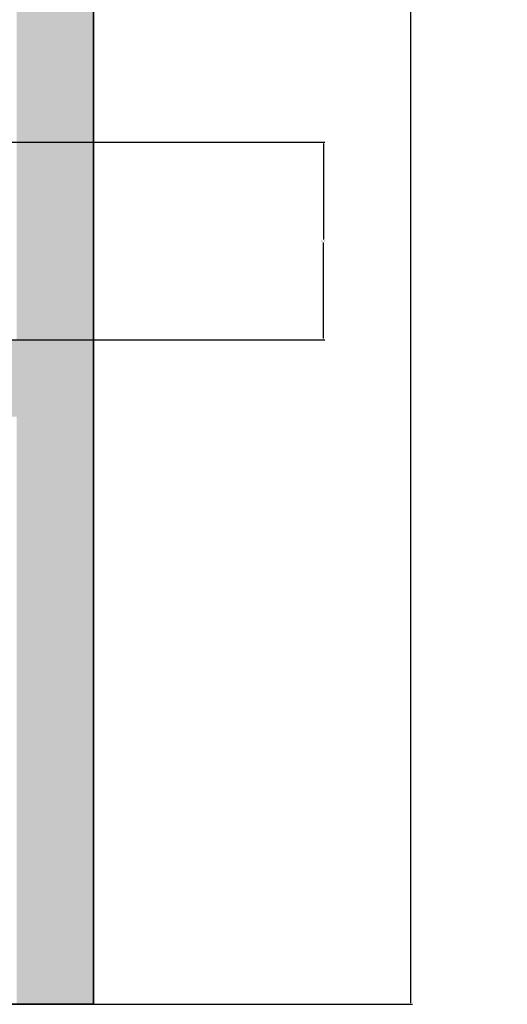
# Model space of a CAD drawing. Units: inches. Extents: x -5 to 330, y -522 to 40.
# Tile 18 of 23: x 272 to 330, y -495 to -380. Entities that reach past the tile are written whole.
import ezdxf

# ---------------------------------------------------------------- set-up
doc = ezdxf.new("R2010")
doc.units = ezdxf.units.IN
doc.header["$MEASUREMENT"] = 0
for name, color, linetype, lineweight in [('A-ANNO-DIMS', 2, 'Continuous', 18), ('A-SITE-WALL', 7, 'Continuous', 35), ('A-WALL', 7, 'Continuous', 35)]:
    doc.layers.add(name, color=color, linetype=linetype, lineweight=lineweight)
doc.layers.add('A-WALL-PATT', color=18, linetype='Continuous', lineweight=13, true_color=0x000000)
doc.styles.get("Standard").update_dxf_attribs({"font": 'arial.ttf'})
doc.dimstyles.get("Standard").update_dxf_attribs({"dimtxt": 0.18, "dimasz": 0.18, "dimexe": 0.18, "dimexo": 0.0625, "dimgap": 0.09, "dimtad": 0, "dimtih": 1, "dimtoh": 1, "dimdec": 0, "dimzin": 0, "dimdsep": 46, "dimlunit": 3, "dimtxsty": 'Standard', "dimcen": 0.09, "dimadec": 0, "dimazin": 0, "dimtfac": 1, "dimtdec": 0, "dimtofl": 0, "dimtmove": 0, "dimatfit": 3, "dimfxl": 1, "dimtolj": 1, "dimtzin": 0, "dimarcsym": 0})

# ---------------------------------------------------------------- blocks, each defined once
blk = doc.blocks.new('*D6')
at = {"layer": 'A-ANNO-DIMS', "color": 0, "lineweight": -2, "transparency": 16777216}
for p, q in [((281.07, 12.36), (318.43, 12.36)), ((318.25, 12.18), (318.25, -238.29)), ((318.25, -494.96), (318.25, -244.5)), ((281.07, -495.14), (318.43, -495.14))]:
    blk.add_line(p, q, dxfattribs=at)
at = {"layer": 'A-ANNO-DIMS', "color": 0, "transparency": 16777216}
for points in [[(318.22, 12.18), (318.28, 12.18), (318.25, 12.36)], [(318.22, -494.96), (318.28, -494.96), (318.25, -495.14)]]:
    blk.add_solid(points, dxfattribs=at)
at = {"layer": 'Defpoints', "color": 0, "transparency": 16777216}
for p in [(281.01, 12.36), (281.01, -495.14), (318.25, -495.14)]:
    blk.add_point(p, dxfattribs=at)
at = {"layer": 'A-ANNO-DIMS', "color": 0, "transparency": 16777216, "insert": (318.25, -241.39), "char_height": 6, "attachment_point": 5}
blk.add_mtext('\\A1;42\'-4"', dxfattribs=at)
blk = doc.blocks.new('*D44')
at = {"layer": 'A-ANNO-DIMS', "color": 0, "lineweight": -2, "transparency": 16777216}
for p, q in [((128.57, -393.93), (308.17, -393.93)), ((307.99, -394.11), (307.99, -405.36)), ((307.99, -416.96), (307.99, -405.72)), ((128.57, -417.14), (308.17, -417.14))]:
    blk.add_line(p, q, dxfattribs=at)
at = {"layer": 'A-ANNO-DIMS', "color": 0, "transparency": 16777216}
for points in [[(307.96, -394.11), (308.02, -394.11), (307.99, -393.93)], [(307.96, -416.96), (308.02, -416.96), (307.99, -417.14)]]:
    blk.add_solid(points, dxfattribs=at)
at = {"layer": 'Defpoints', "color": 0, "transparency": 16777216}
for p in [(128.51, -393.93), (307.99, -393.93), (128.51, -417.14)]:
    blk.add_point(p, dxfattribs=at)
at = {"layer": 'A-ANNO-DIMS', "color": 0, "transparency": 16777216, "insert": (307.99, -405.54), "char_height": 0.18, "attachment_point": 5}
blk.add_mtext('\\A1;1\'-11"', dxfattribs=at)

msp = doc.modelspace()

# ---------------------------------------------------------------- hatches: boundary and pattern name
at = {"layer": 'A-WALL-PATT'}
h = msp.add_hatch(color=256, dxfattribs=at)
h.dxf.hatch_style = 1
h.paths.add_polyline_path([(164.01, -44.15), (159.51, -44.15), (159.51, -153.14), (164.01, -153.14)], flags=17)
h.paths.add_polyline_path([(224.01, -188.14), (272.01, -188.14), (272.01, -218.14), (260.01, -218.14), (260.01, -222.64), (272.01, -222.64), (272.01, -292.64), (159.01, -292.64), (159.01, -297.14), (272.01, -297.14), (272.01, -417.14), (245.51, -417.14), (245.51, -426.14), (272.01, -426.14), (272.01, -495.14), (281.01, -495.14), (281.01, 12.36), (23.51, 12.36), (23.51, -426.14), (62.92, -426.14), (62.92, -417.14), (32.51, -417.14), (32.51, -297.14), (48.13, -297.14), (48.13, -292.64), (32.51, -292.64), (32.51, -140.64), (133.51, -140.64), (133.51, -131.64), (32.51, -131.64), (32.51, 3.36), (159.51, 3.36), (164.01, 3.36), (220.01, 3.36), (224.51, 3.36), (272.01, 3.36), (272.01, -179.14), (159.51, -179.14), (159.51, -188.14), (219.51, -188.14), (219.51, -266.64), (224.01, -266.64), (224.01, -222.64), (236.01, -222.64), (236.01, -218.14), (224.01, -218.14)])
h.paths.add_polyline_path([(133.01, -292.64), (128.51, -292.64), (128.51, -297.14), (128.51, -417.14), (122.92, -417.14), (122.92, -426.14), (133.01, -426.14)], flags=17)
h.paths.add_polyline_path([(185.51, -417.14), (159.01, -417.14), (159.01, -426.14), (185.51, -426.14)], flags=17)
h.paths.add_polyline_path([(133.51, -140.64), (129.01, -140.64), (129.01, -246.64), (133.51, -246.64)], flags=17)
h.paths.add_polyline_path([(246.01, -48.64), (224.51, -48.64), (224.51, -27.63), (220.01, -27.63), (220.01, -48.64), (198.6, -48.64), (198.6, -53.14), (246.01, -53.14)], flags=17)

# ---------------------------------------------------------------- linework, layer by layer
at = {"layer": 'A-SITE-WALL'}
msp.add_line((23.51, -495.14), (281.01, -495.14), dxfattribs=at)
at = {"layer": 'A-WALL'}
msp.add_line((281.01, 12.36), (281.01, -495.14), dxfattribs=at)

# ---------------------------------------------------------------- dimensions: what is measured, and where the dimension line sits
at = {"layer": 'A-ANNO-DIMS'}
for base, p1, p2, override, picture, middle in [((318.24603734, -495.14358203), (281.00988858, 12.35641797), (281.00988858, -495.14358203), {"dimtxt": 6, "dimclrd": 0, "dimclre": 0, "dimclrt": 0}, '*D6', (318.24603734, -241.39358203)), ((307.99, -393.93), (128.51, -417.14), (128.51, -393.93), {"dimdec": 1, "dimlfac": 1, "dimrnd": 0, "dimzin": 1, "dimdsep": 46, "dimlunit": 4, "dimfrac": 2}, '*D44', (307.99, -405.54))]:
    dim = msp.add_linear_dim(base=base, p1=p1, p2=p2, angle=90, dimstyle='Standard', override=override, dxfattribs=at)
    dim.commit()
    dim.dimension.update_dxf_attribs({"geometry": picture, "text_midpoint": middle})

doc.saveas('drawing.dxf')
